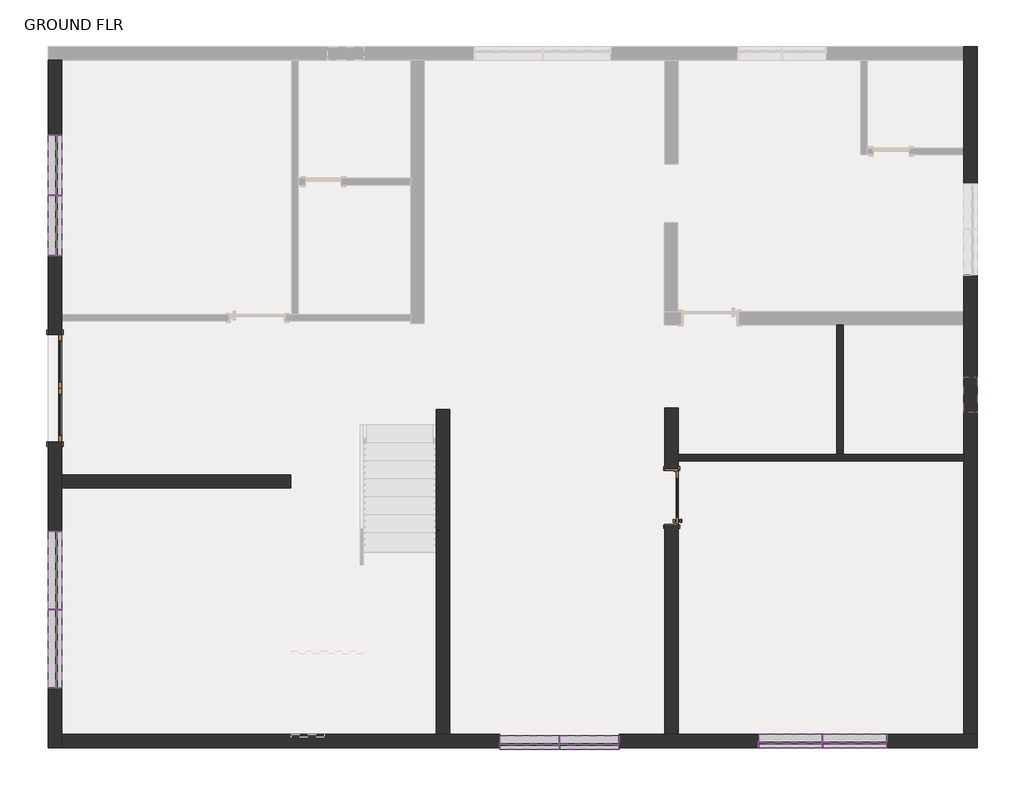
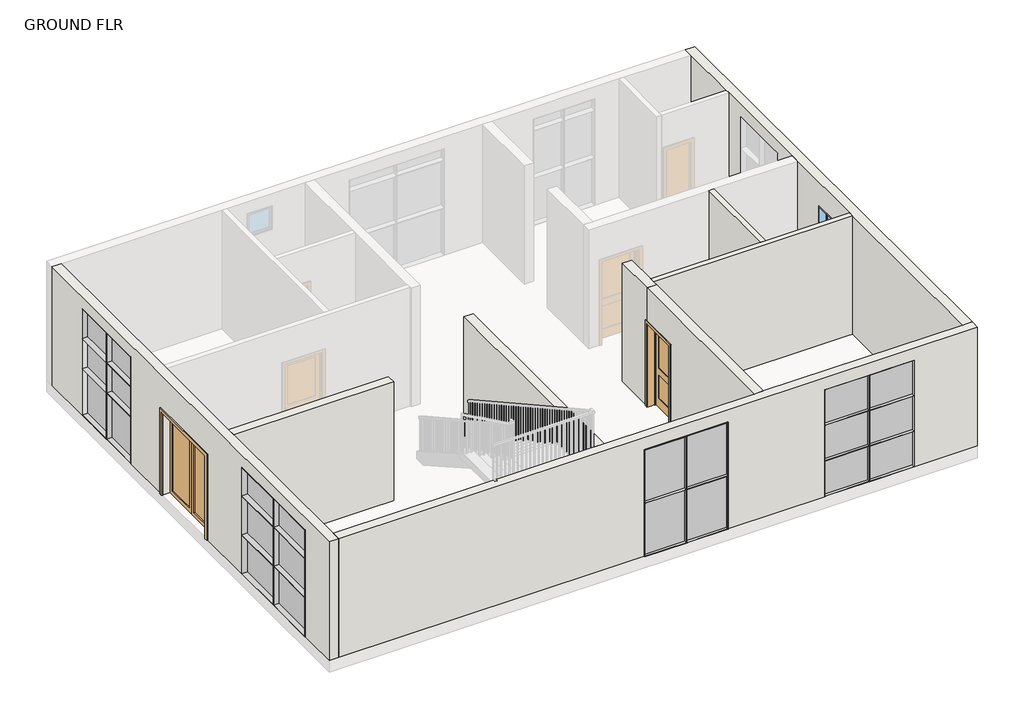
# One storey, part 1 of 3: 61 members, 22 plates, 9 walls, 2 doors, 1 window.
"""IFC4 building model written with IfcOpenShell, lengths in millimetres."""

from ifc_helpers import new_model, si_unit, frame, origin, place, context, project, spatial, polyline, outline, extrude, faceted_brep, transform, mapped, element, save
from components import door_5cbd26dd, door_interior_single_2_panel_wood_5dd36918, member_897fe9bb, member_9b8c6d2b, member_2938acba, member_330b65be, member_3bd50dc0, member_3448d7e6, member_1c5a217c, member_cd12fca0, member_0b5c0894, member_065c0f10, member_eaa18777, member_15c0e2f7, member_46601aaa, member_1d4720dc, member_9e0b9b87, member_6fc4240e, member_2d61f393, member_06a73730, member_9004b0e6, member_781c77f6, system_panel_glazed_9c96ef9a, system_panel_glazed_c3157265, system_panel_glazed_1bc24549, system_panel_glazed_9cc9ac89, system_panel_glazed_cb69acbc, system_panel_glazed_51d5fa28, system_panel_glazed_d128e385, system_panel_glazed_c2edcddf, system_panel_glazed_7a42c5f5, window_80340324

model = new_model("IFC4")

# Units and contexts
model_context = context("Model", 3, world=origin())
ifc_project = project(units=[si_unit("LENGTHUNIT", "METRE", prefix="MILLI")], contexts=[model_context])

# Site, building, storey
site = spatial("IfcSite", under=ifc_project)
building = spatial("IfcBuilding", under=site)
storey = spatial("IfcBuildingStorey", under=building, Name="GROUND FLR", Elevation=304.8)

# Doors
placement = place(None, origin())
door_shape = door_5cbd26dd(model_context)
element("IfcDoor", 1, ObjectType="Door-Double-Glass : 72\" x 84\"", at=placement, inside=storey, context=model_context, shape_type="MappedRepresentation", body=[
    mapped(door_shape, transform((-10241.447001, -123.3828332, 304.8), x_axis=(0.0, -1.0, 0.0), y_axis=(1.0, 0.0, 0.0), z_axis=(0.0, 0.0, 1.0))),
])
door_interior_single_2_panel_wood_shape = door_interior_single_2_panel_wood_5dd36918(model_context)
element("IfcDoor", 2, ObjectType="Door-Interior-Single-2_Panel-Wood", at=placement, inside=storey, context=model_context, shape_type="MappedRepresentation", body=[
    mapped(door_interior_single_2_panel_wood_shape, transform((226.2108119, -1978.5424275, 304.8), x_axis=(0.0, 1.0, 0.0), y_axis=(-1.0, 0.0, 0.0), z_axis=(0.0, 0.0, 1.0))),
])

# Members
member_shape = member_897fe9bb(model_context)
element("IfcMember", 3, ObjectType="Rectangular Mullion : 2.5\" x 5\" rectangular", at=placement, inside=storey, context=model_context, shape_type="MappedRepresentation", body=[
    mapped(member_shape, transform((-10239.065751, 3150.98206, 304.8), x_axis=(0.0, -1.0, 0.0), y_axis=(-1.0, 0.0, 0.0), z_axis=(0.0, 0.0, -1.0))),
])
member_2_shape = member_9b8c6d2b(model_context)
element("IfcMember", 4, ObjectType="Rectangular Mullion : 2.5\" x 5\" rectangular", at=placement, inside=storey, context=model_context, shape_type="MappedRepresentation", body=[
    mapped(member_2_shape, transform((-10239.065751, 2122.28206, 304.8), x_axis=(0.0, -1.0, 0.0), y_axis=(-1.0, 0.0, 0.0), z_axis=(0.0, 0.0, -1.0))),
])
member_3_shape = member_2938acba(model_context)
element("IfcMember", 5, ObjectType="Rectangular Mullion : 2.5\" x 5\" rectangular", at=placement, inside=storey, context=model_context, shape_type="MappedRepresentation", body=[
    mapped(member_3_shape, transform((-10239.065751, 3150.98206, 1498.6), x_axis=(0.0, -1.0, 0.0), y_axis=(-1.0, 0.0, 0.0), z_axis=(0.0, 0.0, -1.0))),
])
element("IfcMember", 6, ObjectType="Rectangular Mullion : 2.5\" x 5\" rectangular", at=placement, inside=storey, context=model_context, shape_type="MappedRepresentation", body=[
    mapped(member_3_shape, transform((-10239.065751, 3150.98206, 2273.3), x_axis=(0.0, -1.0, 0.0), y_axis=(-1.0, 0.0, 0.0), z_axis=(0.0, 0.0, -1.0))),
])
member_4_shape = member_330b65be(model_context)
element("IfcMember", 7, ObjectType="Rectangular Mullion : 2.5\" x 5\" rectangular", at=placement, inside=storey, context=model_context, shape_type="MappedRepresentation", body=[
    mapped(member_4_shape, transform((-10239.065751, 4179.68206, 3048.0), x_axis=(0.0, 1.0, 0.0), y_axis=(-1.0, 0.0, 0.0), z_axis=(0.0, 0.0, 1.0))),
])
element("IfcMember", 8, ObjectType="Rectangular Mullion : 2.5\" x 5\" rectangular", at=placement, inside=storey, context=model_context, shape_type="MappedRepresentation", body=[
    mapped(member_4_shape, transform((-10239.065751, 2122.28206, 1498.6), x_axis=(0.0, -1.0, 0.0), y_axis=(-1.0, 0.0, 0.0), z_axis=(0.0, 0.0, -1.0))),
])
element("IfcMember", 9, ObjectType="Rectangular Mullion : 2.5\" x 5\" rectangular", at=placement, inside=storey, context=model_context, shape_type="MappedRepresentation", body=[
    mapped(member_4_shape, transform((-10239.065751, 2122.28206, 2273.3), x_axis=(0.0, -1.0, 0.0), y_axis=(-1.0, 0.0, 0.0), z_axis=(0.0, 0.0, -1.0))),
])
member_5_shape = member_3bd50dc0(model_context)
element("IfcMember", 10, ObjectType="Rectangular Mullion : 2.5\" x 5\" rectangular", at=placement, inside=storey, context=model_context, shape_type="MappedRepresentation", body=[
    mapped(member_5_shape, transform((-10239.065751, -3879.168209, 2311.4), x_axis=(0.0, -1.0, 0.0), y_axis=(-1.0, 0.0, 0.0), z_axis=(0.0, 0.0, -1.0))),
])
member_6_shape = member_3448d7e6(model_context)
element("IfcMember", 11, ObjectType="Rectangular Mullion : 2.5\" x 5\" rectangular", at=placement, inside=storey, context=model_context, shape_type="MappedRepresentation", body=[
    mapped(member_6_shape, transform((-10239.065751, -2545.668209, 3048.0), x_axis=(0.0, 1.0, 0.0), y_axis=(-1.0, 0.0, 0.0), z_axis=(0.0, 0.0, 1.0))),
])
element("IfcMember", 12, ObjectType="Rectangular Mullion : 2.5\" x 5\" rectangular", at=placement, inside=storey, context=model_context, shape_type="MappedRepresentation", body=[
    mapped(member_6_shape, transform((-10239.065751, -5212.668209, 2311.4), x_axis=(0.0, -1.0, 0.0), y_axis=(-1.0, 0.0, 0.0), z_axis=(0.0, 0.0, -1.0))),
])
member_7_shape = member_1c5a217c(model_context)
element("IfcMember", 13, ObjectType="Rectangular Mullion : 2.5\" x 5\" rectangular", at=placement, inside=storey, context=model_context, shape_type="MappedRepresentation", body=[
    mapped(member_7_shape, transform((-10239.065751, -3879.168209, 304.8), x_axis=(0.0, -1.0, 0.0), y_axis=(-1.0, 0.0, 0.0), z_axis=(0.0, 0.0, -1.0))),
])
element("IfcMember", 14, ObjectType="Rectangular Mullion : 2.5\" x 5\" rectangular", at=placement, inside=storey, context=model_context, shape_type="MappedRepresentation", body=[
    mapped(member_7_shape, transform((-10239.065751, -3879.168209, 1308.1), x_axis=(0.0, -1.0, 0.0), y_axis=(-1.0, 0.0, 0.0), z_axis=(0.0, 0.0, -1.0))),
])
member_8_shape = member_cd12fca0(model_context)
element("IfcMember", 15, ObjectType="Rectangular Mullion : 2.5\" x 5\" rectangular", at=placement, inside=storey, context=model_context, shape_type="MappedRepresentation", body=[
    mapped(member_8_shape, transform((-10239.065751, -5212.668209, 304.8), x_axis=(0.0, -1.0, 0.0), y_axis=(-1.0, 0.0, 0.0), z_axis=(0.0, 0.0, -1.0))),
])
element("IfcMember", 16, ObjectType="Rectangular Mullion : 2.5\" x 5\" rectangular", at=placement, inside=storey, context=model_context, shape_type="MappedRepresentation", body=[
    mapped(member_8_shape, transform((-10239.065751, -2545.668209, 2311.4), x_axis=(0.0, 1.0, 0.0), y_axis=(-1.0, 0.0, 0.0), z_axis=(0.0, 0.0, 1.0))),
])
element("IfcMember", 17, ObjectType="Rectangular Mullion : 2.5\" x 5\" rectangular", at=placement, inside=storey, context=model_context, shape_type="MappedRepresentation", body=[
    mapped(member_8_shape, transform((-10239.065751, -5212.668209, 1308.1), x_axis=(0.0, -1.0, 0.0), y_axis=(-1.0, 0.0, 0.0), z_axis=(0.0, 0.0, -1.0))),
])
element("IfcMember", 18, ObjectType="Rectangular Mullion : 2.5\" x 5\" rectangular", at=placement, inside=storey, context=model_context, shape_type="MappedRepresentation", body=[
    mapped(member_8_shape, transform((-10239.065751, -2545.668209, 1308.1), x_axis=(0.0, 1.0, 0.0), y_axis=(-1.0, 0.0, 0.0), z_axis=(0.0, 0.0, 1.0))),
])
member_9_shape = member_0b5c0894(model_context)
element("IfcMember", 19, ObjectType="Rectangular Mullion : 2.5\" x 5\" rectangular", at=placement, inside=storey, context=model_context, shape_type="MappedRepresentation", body=[
    mapped(member_9_shape, transform((2781.5067356, -6110.4053142, 2133.6), x_axis=(-1.0, 0.0, 0.0), y_axis=(0.0, 1.0, 0.0), z_axis=(0.0, 0.0, -1.0))),
])
member_10_shape = member_065c0f10(model_context)
element("IfcMember", 20, ObjectType="Rectangular Mullion : 2.5\" x 5\" rectangular", at=placement, inside=storey, context=model_context, shape_type="MappedRepresentation", body=[
    mapped(member_10_shape, transform((3873.7067356, -6110.4053142, 3048.0), x_axis=(1.0, 0.0, 0.0), y_axis=(0.0, 1.0, 0.0), z_axis=(0.0, 0.0, 1.0))),
])
element("IfcMember", 21, ObjectType="Rectangular Mullion : 2.5\" x 5\" rectangular", at=placement, inside=storey, context=model_context, shape_type="MappedRepresentation", body=[
    mapped(member_10_shape, transform((1689.3067356, -6110.4053142, 2133.6), x_axis=(-1.0, 0.0, 0.0), y_axis=(0.0, 1.0, 0.0), z_axis=(0.0, 0.0, -1.0))),
])
element("IfcMember", 22, ObjectType="Rectangular Mullion : 2.5\" x 5\" rectangular", at=placement, inside=storey, context=model_context, shape_type="MappedRepresentation", body=[
    mapped(member_9_shape, transform((2781.5067356, -6110.4053142, 304.8), x_axis=(-1.0, 0.0, 0.0), y_axis=(0.0, 1.0, 0.0), z_axis=(0.0, 0.0, -1.0))),
])
element("IfcMember", 23, ObjectType="Rectangular Mullion : 2.5\" x 5\" rectangular", at=placement, inside=storey, context=model_context, shape_type="MappedRepresentation", body=[
    mapped(member_9_shape, transform((2781.5067356, -6110.4053142, 1219.2), x_axis=(-1.0, 0.0, 0.0), y_axis=(0.0, 1.0, 0.0), z_axis=(0.0, 0.0, -1.0))),
])
element("IfcMember", 24, ObjectType="Rectangular Mullion : 2.5\" x 5\" rectangular", at=placement, inside=storey, context=model_context, shape_type="MappedRepresentation", body=[
    mapped(member_10_shape, transform((1689.3067356, -6110.4053142, 304.8), x_axis=(-1.0, 0.0, 0.0), y_axis=(0.0, 1.0, 0.0), z_axis=(0.0, 0.0, -1.0))),
])
element("IfcMember", 25, ObjectType="Rectangular Mullion : 2.5\" x 5\" rectangular", at=placement, inside=storey, context=model_context, shape_type="MappedRepresentation", body=[
    mapped(member_10_shape, transform((3873.7067356, -6110.4053142, 2133.6), x_axis=(1.0, 0.0, 0.0), y_axis=(0.0, 1.0, 0.0), z_axis=(0.0, 0.0, 1.0))),
])
element("IfcMember", 26, ObjectType="Rectangular Mullion : 2.5\" x 5\" rectangular", at=placement, inside=storey, context=model_context, shape_type="MappedRepresentation", body=[
    mapped(member_10_shape, transform((1689.3067356, -6110.4053142, 1219.2), x_axis=(-1.0, 0.0, 0.0), y_axis=(0.0, 1.0, 0.0), z_axis=(0.0, 0.0, -1.0))),
])
element("IfcMember", 27, ObjectType="Rectangular Mullion : 2.5\" x 5\" rectangular", at=placement, inside=storey, context=model_context, shape_type="MappedRepresentation", body=[
    mapped(member_10_shape, transform((3873.7067356, -6110.4053142, 1219.2), x_axis=(1.0, 0.0, 0.0), y_axis=(0.0, 1.0, 0.0), z_axis=(0.0, 0.0, 1.0))),
])
member_11_shape = member_eaa18777(model_context)
element("IfcMember", 28, ObjectType="Rectangular Mullion : 2.5\" x 5\" rectangular", at=placement, inside=storey, context=model_context, shape_type="MappedRepresentation", body=[
    mapped(member_11_shape, transform((-1680.5487435, -6133.1318323, 304.8), x_axis=(-1.0, 0.0, 0.0), y_axis=(0.0, 1.0, 0.0), z_axis=(0.0, 0.0, -1.0))),
])
element("IfcMember", 29, ObjectType="Rectangular Mullion : 2.5\" x 5\" rectangular", at=placement, inside=storey, context=model_context, shape_type="MappedRepresentation", body=[
    mapped(member_11_shape, transform((-1680.5487435, -6133.1318323, 1676.4), x_axis=(-1.0, 0.0, 0.0), y_axis=(0.0, 1.0, 0.0), z_axis=(0.0, 0.0, -1.0))),
])
member_12_shape = member_15c0e2f7(model_context)
element("IfcMember", 30, ObjectType="Rectangular Mullion : 2.5\" x 5\" rectangular", at=placement, inside=storey, context=model_context, shape_type="MappedRepresentation", body=[
    mapped(member_12_shape, transform((-2696.5487435, -6133.1318323, 304.8), x_axis=(-1.0, 0.0, 0.0), y_axis=(0.0, 1.0, 0.0), z_axis=(0.0, 0.0, -1.0))),
])
element("IfcMember", 31, ObjectType="Rectangular Mullion : 2.5\" x 5\" rectangular", at=placement, inside=storey, context=model_context, shape_type="MappedRepresentation", body=[
    mapped(member_12_shape, transform((-664.5487435, -6133.1318323, 3048.0), x_axis=(1.0, 0.0, 0.0), y_axis=(0.0, 1.0, 0.0), z_axis=(0.0, 0.0, 1.0))),
])
element("IfcMember", 32, ObjectType="Rectangular Mullion : 2.5\" x 5\" rectangular", at=placement, inside=storey, context=model_context, shape_type="MappedRepresentation", body=[
    mapped(member_12_shape, transform((-2696.5487435, -6133.1318323, 1676.4), x_axis=(-1.0, 0.0, 0.0), y_axis=(0.0, 1.0, 0.0), z_axis=(0.0, 0.0, -1.0))),
])
element("IfcMember", 33, ObjectType="Rectangular Mullion : 2.5\" x 5\" rectangular", at=placement, inside=storey, context=model_context, shape_type="MappedRepresentation", body=[
    mapped(member_12_shape, transform((-664.5487435, -6133.1318323, 1676.4), x_axis=(1.0, 0.0, 0.0), y_axis=(0.0, 1.0, 0.0), z_axis=(0.0, 0.0, 1.0))),
])
member_13_shape = member_46601aaa(model_context)
element("IfcMember", 34, ObjectType="Rectangular Mullion : 2.5\" x 5\" rectangular", at=placement, inside=storey, context=model_context, shape_type="MappedRepresentation", body=[
    mapped(member_13_shape, transform((-10239.065751, 2129.52106, 3048.0), x_axis=(0.0, 0.0, 1.0), y_axis=(-1.0, 0.0, 0.0), z_axis=(0.0, -1.0, 0.0))),
])
element("IfcMember", 35, ObjectType="Rectangular Mullion : 2.5\" x 5\" rectangular", at=placement, inside=storey, context=model_context, shape_type="MappedRepresentation", body=[
    mapped(member_13_shape, transform((-10239.065751, 3154.60156, 3048.0), x_axis=(0.0, 0.0, 1.0), y_axis=(-1.0, 0.0, 0.0), z_axis=(0.0, -1.0, 0.0))),
])
element("IfcMember", 36, ObjectType="Rectangular Mullion : 2.5\" x 5\" rectangular", at=placement, inside=storey, context=model_context, shape_type="MappedRepresentation", body=[
    mapped(member_13_shape, transform((-10239.065751, 4172.44306, 304.8), x_axis=(0.0, 0.0, -1.0), y_axis=(-1.0, 0.0, 0.0), z_axis=(0.0, 1.0, 0.0))),
])
element("IfcMember", 37, ObjectType="Rectangular Mullion : 2.5\" x 5\" rectangular", at=placement, inside=storey, context=model_context, shape_type="MappedRepresentation", body=[
    mapped(member_13_shape, transform((-10239.065751, 3147.36256, 304.8), x_axis=(0.0, 0.0, -1.0), y_axis=(-1.0, 0.0, 0.0), z_axis=(0.0, 1.0, 0.0))),
])
member_14_shape = member_1d4720dc(model_context)
element("IfcMember", 38, ObjectType="Rectangular Mullion : 2.5\" x 5\" rectangular", at=placement, inside=storey, context=model_context, shape_type="MappedRepresentation", body=[
    mapped(member_14_shape, transform((-10239.065751, 3154.60156, 1498.6), x_axis=(0.0, 0.0, 1.0), y_axis=(-1.0, 0.0, 0.0), z_axis=(0.0, -1.0, 0.0))),
])
element("IfcMember", 39, ObjectType="Rectangular Mullion : 2.5\" x 5\" rectangular", at=placement, inside=storey, context=model_context, shape_type="MappedRepresentation", body=[
    mapped(member_14_shape, transform((-10239.065751, 2129.52106, 1498.6), x_axis=(0.0, 0.0, 1.0), y_axis=(-1.0, 0.0, 0.0), z_axis=(0.0, -1.0, 0.0))),
])
element("IfcMember", 40, ObjectType="Rectangular Mullion : 2.5\" x 5\" rectangular", at=placement, inside=storey, context=model_context, shape_type="MappedRepresentation", body=[
    mapped(member_14_shape, transform((-10239.065751, 3154.60156, 2273.3), x_axis=(0.0, 0.0, 1.0), y_axis=(-1.0, 0.0, 0.0), z_axis=(0.0, -1.0, 0.0))),
])
element("IfcMember", 41, ObjectType="Rectangular Mullion : 2.5\" x 5\" rectangular", at=placement, inside=storey, context=model_context, shape_type="MappedRepresentation", body=[
    mapped(member_14_shape, transform((-10239.065751, 2129.52106, 2273.3), x_axis=(0.0, 0.0, 1.0), y_axis=(-1.0, 0.0, 0.0), z_axis=(0.0, -1.0, 0.0))),
])
member_15_shape = member_9e0b9b87(model_context)
element("IfcMember", 42, ObjectType="Rectangular Mullion : 2.5\" x 5\" rectangular", at=placement, inside=storey, context=model_context, shape_type="MappedRepresentation", body=[
    mapped(member_15_shape, transform((-10239.065751, -5205.429209, 3048.0), x_axis=(0.0, 0.0, 1.0), y_axis=(-1.0, 0.0, 0.0), z_axis=(0.0, -1.0, 0.0))),
])
element("IfcMember", 43, ObjectType="Rectangular Mullion : 2.5\" x 5\" rectangular", at=placement, inside=storey, context=model_context, shape_type="MappedRepresentation", body=[
    mapped(member_15_shape, transform((-10239.065751, -3875.548709, 3048.0), x_axis=(0.0, 0.0, 1.0), y_axis=(-1.0, 0.0, 0.0), z_axis=(0.0, -1.0, 0.0))),
])
element("IfcMember", 44, ObjectType="Rectangular Mullion : 2.5\" x 5\" rectangular", at=placement, inside=storey, context=model_context, shape_type="MappedRepresentation", body=[
    mapped(member_15_shape, transform((-10239.065751, -2552.907209, 304.8), x_axis=(0.0, 0.0, -1.0), y_axis=(-1.0, 0.0, 0.0), z_axis=(0.0, 1.0, 0.0))),
])
element("IfcMember", 45, ObjectType="Rectangular Mullion : 2.5\" x 5\" rectangular", at=placement, inside=storey, context=model_context, shape_type="MappedRepresentation", body=[
    mapped(member_15_shape, transform((-10239.065751, -3882.787709, 304.8), x_axis=(0.0, 0.0, -1.0), y_axis=(-1.0, 0.0, 0.0), z_axis=(0.0, 1.0, 0.0))),
])
member_16_shape = member_6fc4240e(model_context)
element("IfcMember", 46, ObjectType="Rectangular Mullion : 2.5\" x 5\" rectangular", at=placement, inside=storey, context=model_context, shape_type="MappedRepresentation", body=[
    mapped(member_16_shape, transform((-10239.065751, -3875.548709, 2311.4), x_axis=(0.0, 0.0, 1.0), y_axis=(-1.0, 0.0, 0.0), z_axis=(0.0, -1.0, 0.0))),
])
element("IfcMember", 47, ObjectType="Rectangular Mullion : 2.5\" x 5\" rectangular", at=placement, inside=storey, context=model_context, shape_type="MappedRepresentation", body=[
    mapped(member_16_shape, transform((-10239.065751, -5205.429209, 2311.4), x_axis=(0.0, 0.0, 1.0), y_axis=(-1.0, 0.0, 0.0), z_axis=(0.0, -1.0, 0.0))),
])
element("IfcMember", 48, ObjectType="Rectangular Mullion : 2.5\" x 5\" rectangular", at=placement, inside=storey, context=model_context, shape_type="MappedRepresentation", body=[
    mapped(member_16_shape, transform((-10239.065751, -3875.548709, 1308.1), x_axis=(0.0, 0.0, 1.0), y_axis=(-1.0, 0.0, 0.0), z_axis=(0.0, -1.0, 0.0))),
])
element("IfcMember", 49, ObjectType="Rectangular Mullion : 2.5\" x 5\" rectangular", at=placement, inside=storey, context=model_context, shape_type="MappedRepresentation", body=[
    mapped(member_16_shape, transform((-10239.065751, -5205.429209, 1308.1), x_axis=(0.0, 0.0, 1.0), y_axis=(-1.0, 0.0, 0.0), z_axis=(0.0, -1.0, 0.0))),
])
member_17_shape = member_2d61f393(model_context)
element("IfcMember", 50, ObjectType="Rectangular Mullion : 2.5\" x 5\" rectangular", at=placement, inside=storey, context=model_context, shape_type="MappedRepresentation", body=[
    mapped(member_17_shape, transform((1696.5457356, -6110.4053142, 3048.0), x_axis=(0.0, 0.0, 1.0), y_axis=(0.0, 1.0, 0.0), z_axis=(-1.0, 0.0, 0.0))),
])
element("IfcMember", 51, ObjectType="Rectangular Mullion : 2.5\" x 5\" rectangular", at=placement, inside=storey, context=model_context, shape_type="MappedRepresentation", body=[
    mapped(member_17_shape, transform((2785.1262356, -6110.4053142, 3048.0), x_axis=(0.0, 0.0, 1.0), y_axis=(0.0, 1.0, 0.0), z_axis=(-1.0, 0.0, 0.0))),
])
element("IfcMember", 52, ObjectType="Rectangular Mullion : 2.5\" x 5\" rectangular", at=placement, inside=storey, context=model_context, shape_type="MappedRepresentation", body=[
    mapped(member_17_shape, transform((3866.4677356, -6110.4053142, 304.8), x_axis=(0.0, 0.0, -1.0), y_axis=(0.0, 1.0, 0.0), z_axis=(1.0, 0.0, 0.0))),
])
element("IfcMember", 53, ObjectType="Rectangular Mullion : 2.5\" x 5\" rectangular", at=placement, inside=storey, context=model_context, shape_type="MappedRepresentation", body=[
    mapped(member_17_shape, transform((2777.8872356, -6110.4053142, 304.8), x_axis=(0.0, 0.0, -1.0), y_axis=(0.0, 1.0, 0.0), z_axis=(1.0, 0.0, 0.0))),
])
member_18_shape = member_06a73730(model_context)
element("IfcMember", 54, ObjectType="Rectangular Mullion : 2.5\" x 5\" rectangular", at=placement, inside=storey, context=model_context, shape_type="MappedRepresentation", body=[
    mapped(member_18_shape, transform((2785.1262356, -6110.4053142, 2133.6), x_axis=(0.0, 0.0, 1.0), y_axis=(0.0, 1.0, 0.0), z_axis=(-1.0, 0.0, 0.0))),
])
element("IfcMember", 55, ObjectType="Rectangular Mullion : 2.5\" x 5\" rectangular", at=placement, inside=storey, context=model_context, shape_type="MappedRepresentation", body=[
    mapped(member_18_shape, transform((1696.5457356, -6110.4053142, 2133.6), x_axis=(0.0, 0.0, 1.0), y_axis=(0.0, 1.0, 0.0), z_axis=(-1.0, 0.0, 0.0))),
])
element("IfcMember", 56, ObjectType="Rectangular Mullion : 2.5\" x 5\" rectangular", at=placement, inside=storey, context=model_context, shape_type="MappedRepresentation", body=[
    mapped(member_18_shape, transform((2785.1262356, -6110.4053142, 1219.2), x_axis=(0.0, 0.0, 1.0), y_axis=(0.0, 1.0, 0.0), z_axis=(-1.0, 0.0, 0.0))),
])
element("IfcMember", 57, ObjectType="Rectangular Mullion : 2.5\" x 5\" rectangular", at=placement, inside=storey, context=model_context, shape_type="MappedRepresentation", body=[
    mapped(member_18_shape, transform((1696.5457356, -6110.4053142, 1219.2), x_axis=(0.0, 0.0, 1.0), y_axis=(0.0, 1.0, 0.0), z_axis=(-1.0, 0.0, 0.0))),
])
member_19_shape = member_9004b0e6(model_context)
element("IfcMember", 58, ObjectType="Rectangular Mullion : 2.5\" x 5\" rectangular", at=placement, inside=storey, context=model_context, shape_type="MappedRepresentation", body=[
    mapped(member_19_shape, transform((-2689.3097435, -6133.1318323, 3048.0), x_axis=(0.0, 0.0, 1.0), y_axis=(0.0, 1.0, 0.0), z_axis=(-1.0, 0.0, 0.0))),
])
element("IfcMember", 59, ObjectType="Rectangular Mullion : 2.5\" x 5\" rectangular", at=placement, inside=storey, context=model_context, shape_type="MappedRepresentation", body=[
    mapped(member_19_shape, transform((-1676.9292435, -6133.1318323, 3048.0), x_axis=(0.0, 0.0, 1.0), y_axis=(0.0, 1.0, 0.0), z_axis=(-1.0, 0.0, 0.0))),
])
element("IfcMember", 60, ObjectType="Rectangular Mullion : 2.5\" x 5\" rectangular", at=placement, inside=storey, context=model_context, shape_type="MappedRepresentation", body=[
    mapped(member_19_shape, transform((-671.7877435, -6133.1318323, 304.8), x_axis=(0.0, 0.0, -1.0), y_axis=(0.0, 1.0, 0.0), z_axis=(1.0, 0.0, 0.0))),
])
element("IfcMember", 61, ObjectType="Rectangular Mullion : 2.5\" x 5\" rectangular", at=placement, inside=storey, context=model_context, shape_type="MappedRepresentation", body=[
    mapped(member_19_shape, transform((-1684.1682435, -6133.1318323, 304.8), x_axis=(0.0, 0.0, -1.0), y_axis=(0.0, 1.0, 0.0), z_axis=(1.0, 0.0, 0.0))),
])
member_20_shape = member_781c77f6(model_context)
element("IfcMember", 62, ObjectType="Rectangular Mullion : 2.5\" x 5\" rectangular", at=placement, inside=storey, context=model_context, shape_type="MappedRepresentation", body=[
    mapped(member_20_shape, transform((-1676.9292435, -6133.1318323, 1676.4), x_axis=(0.0, 0.0, 1.0), y_axis=(0.0, 1.0, 0.0), z_axis=(-1.0, 0.0, 0.0))),
])
element("IfcMember", 63, ObjectType="Rectangular Mullion : 2.5\" x 5\" rectangular", at=placement, inside=storey, context=model_context, shape_type="MappedRepresentation", body=[
    mapped(member_20_shape, transform((-2689.3097435, -6133.1318323, 1676.4), x_axis=(0.0, 0.0, 1.0), y_axis=(0.0, 1.0, 0.0), z_axis=(-1.0, 0.0, 0.0))),
])

# Plates
system_panel_glazed_shape = system_panel_glazed_9c96ef9a(model_context)
element("IfcPlate", 64, ObjectType="System Panel : Glazed", at=placement, inside=storey, context=model_context, shape_type="MappedRepresentation", body=[
    mapped(system_panel_glazed_shape, transform((-10239.065751, 3663.52231, 312.039), x_axis=(0.0, -1.0, 0.0), y_axis=(1.0, 0.0, 0.0), z_axis=(0.0, 0.0, 1.0))),
])
element("IfcPlate", 65, ObjectType="System Panel : Glazed", at=placement, inside=storey, context=model_context, shape_type="MappedRepresentation", body=[
    mapped(system_panel_glazed_shape, transform((-10239.065751, 2638.44181, 312.039), x_axis=(0.0, -1.0, 0.0), y_axis=(1.0, 0.0, 0.0), z_axis=(0.0, 0.0, 1.0))),
])
system_panel_glazed_2_shape = system_panel_glazed_c3157265(model_context)
element("IfcPlate", 66, ObjectType="System Panel : Glazed", at=placement, inside=storey, context=model_context, shape_type="MappedRepresentation", body=[
    mapped(system_panel_glazed_2_shape, transform((-10239.065751, -3214.227959, 312.039), x_axis=(0.0, -1.0, 0.0), y_axis=(1.0, 0.0, 0.0), z_axis=(0.0, 0.0, 1.0))),
])
element("IfcPlate", 67, ObjectType="System Panel : Glazed", at=placement, inside=storey, context=model_context, shape_type="MappedRepresentation", body=[
    mapped(system_panel_glazed_2_shape, transform((-10239.065751, -4544.108459, 312.039), x_axis=(0.0, -1.0, 0.0), y_axis=(1.0, 0.0, 0.0), z_axis=(0.0, 0.0, 1.0))),
])
system_panel_glazed_3_shape = system_panel_glazed_1bc24549(model_context)
element("IfcPlate", 68, ObjectType="System Panel : Glazed", at=placement, inside=storey, context=model_context, shape_type="MappedRepresentation", body=[
    mapped(system_panel_glazed_3_shape, transform((3325.7969856, -6110.4053142, 312.039), x_axis=(-1.0, 0.0, 0.0), y_axis=(0.0, -1.0, 0.0), z_axis=(0.0, 0.0, 1.0))),
])
element("IfcPlate", 69, ObjectType="System Panel : Glazed", at=placement, inside=storey, context=model_context, shape_type="MappedRepresentation", body=[
    mapped(system_panel_glazed_3_shape, transform((2237.2164856, -6110.4053142, 312.039), x_axis=(-1.0, 0.0, 0.0), y_axis=(0.0, -1.0, 0.0), z_axis=(0.0, 0.0, 1.0))),
])
element("IfcPlate", 70, ObjectType="System Panel : Glazed", at=placement, inside=storey, context=model_context, shape_type="MappedRepresentation", body=[
    mapped(system_panel_glazed_3_shape, transform((3325.7969856, -6110.4053142, 2137.2195), x_axis=(-1.0, 0.0, 0.0), y_axis=(0.0, -1.0, 0.0), z_axis=(0.0, 0.0, 1.0))),
])
element("IfcPlate", 71, ObjectType="System Panel : Glazed", at=placement, inside=storey, context=model_context, shape_type="MappedRepresentation", body=[
    mapped(system_panel_glazed_3_shape, transform((2237.2164856, -6110.4053142, 2137.2195), x_axis=(-1.0, 0.0, 0.0), y_axis=(0.0, -1.0, 0.0), z_axis=(0.0, 0.0, 1.0))),
])
system_panel_glazed_4_shape = system_panel_glazed_9cc9ac89(model_context)
element("IfcPlate", 72, ObjectType="System Panel : Glazed", at=placement, inside=storey, context=model_context, shape_type="MappedRepresentation", body=[
    mapped(system_panel_glazed_4_shape, transform((-1174.3584935, -6133.1318323, 312.039), x_axis=(-1.0, 0.0, 0.0), y_axis=(0.0, -1.0, 0.0), z_axis=(0.0, 0.0, 1.0))),
])
element("IfcPlate", 73, ObjectType="System Panel : Glazed", at=placement, inside=storey, context=model_context, shape_type="MappedRepresentation", body=[
    mapped(system_panel_glazed_4_shape, transform((-2186.7389935, -6133.1318323, 312.039), x_axis=(-1.0, 0.0, 0.0), y_axis=(0.0, -1.0, 0.0), z_axis=(0.0, 0.0, 1.0))),
])
element("IfcPlate", 74, ObjectType="System Panel : Glazed", at=placement, inside=storey, context=model_context, shape_type="MappedRepresentation", body=[
    mapped(system_panel_glazed_4_shape, transform((-1174.3584935, -6133.1318323, 1680.0195), x_axis=(-1.0, 0.0, 0.0), y_axis=(0.0, -1.0, 0.0), z_axis=(0.0, 0.0, 1.0))),
])
element("IfcPlate", 75, ObjectType="System Panel : Glazed", at=placement, inside=storey, context=model_context, shape_type="MappedRepresentation", body=[
    mapped(system_panel_glazed_4_shape, transform((-2186.7389935, -6133.1318323, 1680.0195), x_axis=(-1.0, 0.0, 0.0), y_axis=(0.0, -1.0, 0.0), z_axis=(0.0, 0.0, 1.0))),
])
system_panel_glazed_5_shape = system_panel_glazed_cb69acbc(model_context)
element("IfcPlate", 76, ObjectType="System Panel : Glazed", at=placement, inside=storey, context=model_context, shape_type="MappedRepresentation", body=[
    mapped(system_panel_glazed_5_shape, transform((-10239.065751, 3663.52231, 1502.2195), x_axis=(0.0, -1.0, 0.0), y_axis=(1.0, 0.0, 0.0), z_axis=(0.0, 0.0, 1.0))),
])
element("IfcPlate", 77, ObjectType="System Panel : Glazed", at=placement, inside=storey, context=model_context, shape_type="MappedRepresentation", body=[
    mapped(system_panel_glazed_5_shape, transform((-10239.065751, 2638.44181, 1502.2195), x_axis=(0.0, -1.0, 0.0), y_axis=(1.0, 0.0, 0.0), z_axis=(0.0, 0.0, 1.0))),
])
system_panel_glazed_6_shape = system_panel_glazed_51d5fa28(model_context)
element("IfcPlate", 78, ObjectType="System Panel : Glazed", at=placement, inside=storey, context=model_context, shape_type="MappedRepresentation", body=[
    mapped(system_panel_glazed_6_shape, transform((-10239.065751, 3663.52231, 2276.9195), x_axis=(0.0, -1.0, 0.0), y_axis=(1.0, 0.0, 0.0), z_axis=(0.0, 0.0, 1.0))),
])
element("IfcPlate", 79, ObjectType="System Panel : Glazed", at=placement, inside=storey, context=model_context, shape_type="MappedRepresentation", body=[
    mapped(system_panel_glazed_6_shape, transform((-10239.065751, 2638.44181, 2276.9195), x_axis=(0.0, -1.0, 0.0), y_axis=(1.0, 0.0, 0.0), z_axis=(0.0, 0.0, 1.0))),
])
system_panel_glazed_7_shape = system_panel_glazed_d128e385(model_context)
element("IfcPlate", 80, ObjectType="System Panel : Glazed", at=placement, inside=storey, context=model_context, shape_type="MappedRepresentation", body=[
    mapped(system_panel_glazed_7_shape, transform((-10239.065751, -3214.227959, 2315.0195), x_axis=(0.0, -1.0, 0.0), y_axis=(1.0, 0.0, 0.0), z_axis=(0.0, 0.0, 1.0))),
])
element("IfcPlate", 81, ObjectType="System Panel : Glazed", at=placement, inside=storey, context=model_context, shape_type="MappedRepresentation", body=[
    mapped(system_panel_glazed_7_shape, transform((-10239.065751, -4544.108459, 2315.0195), x_axis=(0.0, -1.0, 0.0), y_axis=(1.0, 0.0, 0.0), z_axis=(0.0, 0.0, 1.0))),
])
system_panel_glazed_8_shape = system_panel_glazed_c2edcddf(model_context)
element("IfcPlate", 82, ObjectType="System Panel : Glazed", at=placement, inside=storey, context=model_context, shape_type="MappedRepresentation", body=[
    mapped(system_panel_glazed_8_shape, transform((-10239.065751, -3214.227959, 1311.7195), x_axis=(0.0, -1.0, 0.0), y_axis=(1.0, 0.0, 0.0), z_axis=(0.0, 0.0, 1.0))),
])
element("IfcPlate", 83, ObjectType="System Panel : Glazed", at=placement, inside=storey, context=model_context, shape_type="MappedRepresentation", body=[
    mapped(system_panel_glazed_8_shape, transform((-10239.065751, -4544.108459, 1311.7195), x_axis=(0.0, -1.0, 0.0), y_axis=(1.0, 0.0, 0.0), z_axis=(0.0, 0.0, 1.0))),
])
system_panel_glazed_9_shape = system_panel_glazed_7a42c5f5(model_context)
element("IfcPlate", 84, ObjectType="System Panel : Glazed", at=placement, inside=storey, context=model_context, shape_type="MappedRepresentation", body=[
    mapped(system_panel_glazed_9_shape, transform((3325.7969856, -6110.4053142, 1222.8195), x_axis=(-1.0, 0.0, 0.0), y_axis=(0.0, -1.0, 0.0), z_axis=(0.0, 0.0, 1.0))),
])
element("IfcPlate", 85, ObjectType="System Panel : Glazed", at=placement, inside=storey, context=model_context, shape_type="MappedRepresentation", body=[
    mapped(system_panel_glazed_9_shape, transform((2237.2164856, -6110.4053142, 1222.8195), x_axis=(-1.0, 0.0, 0.0), y_axis=(0.0, -1.0, 0.0), z_axis=(0.0, 0.0, 1.0))),
])

# Walls
element("IfcWall", 86, at=placement, inside=storey, context=model_context, shape_type="Brep", body=[
    faceted_brep([(5407.334249, -6224.7053142, 3352.8), (-10124.765751, -6224.7053142, 3352.8), (-10124.765751, -6224.7053142, 304.8), (-2696.5487435, -6224.7053142, 304.8), (-2696.5487435, -6224.7053142, 3048.0), (-664.5487435, -6224.7053142, 3048.0), (-664.5487435, -6224.7053142, 304.8), (1689.3067356, -6224.7053142, 304.8), (1689.3067356, -6224.7053142, 3048.0), (3873.7067356, -6224.7053142, 3048.0), (3873.7067356, -6224.7053142, 304.8), (5407.334249, -6224.7053142, 304.8), (-10124.765751, -5996.1053142, 3352.8), (-3766.7446058, -5996.1053142, 3352.8), (-3538.1446058, -5996.1053142, 3352.8), (108.7358119, -5996.1053142, 3352.8), (337.3358119, -5996.1053142, 3352.8), (5178.734249, -5996.1053142, 3352.8), (5407.334249, -5996.1053142, 3352.8), (5407.334249, -5996.1053142, 304.8), (5178.734249, -5996.1053142, 304.8), (3873.7067356, -5996.1053142, 304.8), (3873.7067356, -5996.1053142, 3048.0), (1689.3067356, -5996.1053142, 3048.0), (1689.3067356, -5996.1053142, 304.8), (337.3358119, -5996.1053142, 304.8), (108.7358119, -5996.1053142, 304.8), (-664.5487435, -5996.1053142, 304.8), (-664.5487435, -5996.1053142, 3048.0), (-2696.5487435, -5996.1053142, 3048.0), (-2696.5487435, -5996.1053142, 304.8), (-3538.1446058, -5996.1053142, 304.8), (-3766.7446058, -5996.1053142, 304.8), (-10124.765751, -5996.1053142, 304.8)], [[[0, 1, 2, 3, 4, 5, 6, 7, 8, 9, 10, 11]], [[12, 13, 14, 15, 16, 17, 18, 19, 20, 21, 22, 23, 24, 25, 26, 27, 28, 29, 30, 31, 32, 33]], [[19, 11, 10, 21, 20]], [[2, 33, 32, 31, 30, 3]], [[24, 7, 6, 27, 26, 25]], [[1, 0, 18, 17, 16, 15, 14, 13, 12]], [[0, 11, 19, 18]], [[2, 1, 12, 33]], [[9, 22, 21, 10]], [[22, 9, 8, 23]], [[23, 8, 7, 24]], [[5, 28, 27, 6]], [[28, 5, 4, 29]], [[29, 4, 3, 30]]]),
])
element("IfcWall", 87, at=placement, inside=storey, context=model_context, shape_type="Brep", body=[
    faceted_brep([(5407.334249, 5675.1946858, 3352.8), (5407.334249, -5996.1053142, 3352.8), (5407.334249, -5996.1053142, 304.8), (5407.334249, 1793.1596634, 304.8), (5407.334249, 1793.1596634, 3048.0), (5407.334249, 3348.9096634, 3048.0), (5407.334249, 3348.9096634, 304.8), (5407.334249, 5675.1946858, 304.8), (5407.334249, -538.3216798, 2743.2), (5407.334249, 71.2783202, 2743.2), (5407.334249, 71.2783202, 2133.6), (5407.334249, -538.3216798, 2133.6), (5178.734249, -5996.1053142, 3352.8), (5178.734249, -1357.4716798, 3352.8), (5178.734249, -1243.1716798, 3352.8), (5178.734249, 952.1551442, 3352.8), (5178.734249, 1180.7551442, 3352.8), (5178.734249, 3840.0446858, 3352.8), (5178.734249, 3954.3446858, 3352.8), (5178.734249, 5446.5946858, 3352.8), (5178.734249, 5675.1946858, 3352.8), (5178.734249, 5675.1946858, 304.8), (5178.734249, 5446.5946858, 304.8), (5178.734249, 3954.3446858, 304.8), (5178.734249, 3840.0446858, 304.8), (5178.734249, 3348.9096634, 304.8), (5178.734249, 3348.9096634, 3048.0), (5178.734249, 1793.1596634, 3048.0), (5178.734249, 1793.1596634, 304.8), (5178.734249, 1180.7551442, 304.8), (5178.734249, 952.1551442, 304.8), (5178.734249, -1243.1716798, 304.8), (5178.734249, -1357.4716798, 304.8), (5178.734249, -5996.1053142, 304.8), (5178.734249, -538.3216798, 2743.2), (5178.734249, -538.3216798, 2133.6), (5178.734249, 71.2783202, 2133.6), (5178.734249, 71.2783202, 2743.2)], [[[0, 1, 2, 3, 4, 5, 6, 7], [8, 9, 10, 11]], [[12, 13, 14, 15, 16, 17, 18, 19, 20, 21, 22, 23, 24, 25, 26, 27, 28, 29, 30, 31, 32, 33], [34, 35, 36, 37]], [[2, 33, 32, 31, 30, 29, 28, 3]], [[21, 7, 6, 25, 24, 23, 22]], [[1, 0, 20, 19, 18, 17, 16, 15, 14, 13, 12]], [[2, 1, 12, 33]], [[0, 7, 21, 20]], [[5, 26, 25, 6]], [[26, 5, 4, 27]], [[27, 4, 3, 28]], [[35, 34, 8, 11]], [[36, 35, 11, 10]], [[37, 36, 10, 9]], [[34, 37, 9, 8]]]),
])
element("IfcWall", 88, at=placement, inside=storey, context=model_context, shape_type="Brep", body=[
    faceted_brep([(-10353.365751, -1037.7828332, 2438.4), (-10353.365751, -1037.7828332, 304.8), (-10353.365751, -2545.668209, 304.8), (-10353.365751, -2545.668209, 3048.0), (-10353.365751, -5212.668209, 3048.0), (-10353.365751, -5212.668209, 304.8), (-10353.365751, -6224.7053142, 304.8), (-10353.365751, -6224.7053142, 3352.8), (-10353.365751, 5446.5946858, 3352.8), (-10353.365751, 5446.5946858, 304.8), (-10353.365751, 4179.68206, 304.8), (-10353.365751, 4179.68206, 3048.0), (-10353.365751, 2122.28206, 3048.0), (-10353.365751, 2122.28206, 304.8), (-10353.365751, 791.0171668, 304.8), (-10353.365751, 791.0171668, 2438.4), (-10124.765751, -2545.668209, 304.8), (-10124.765751, -1818.9707851, 304.8), (-10124.765751, -1590.3707851, 304.8), (-10124.765751, -1037.7828332, 304.8), (-10124.765751, -1037.7828332, 2438.4), (-10124.765751, 791.0171668, 2438.4), (-10124.765751, 791.0171668, 304.8), (-10124.765751, 1013.2671668, 304.8), (-10124.765751, 1127.5671668, 304.8), (-10124.765751, 2122.28206, 304.8), (-10124.765751, 2122.28206, 3048.0), (-10124.765751, 4179.68206, 3048.0), (-10124.765751, 4179.68206, 304.8), (-10124.765751, 5446.5946858, 304.8), (-10124.765751, 5446.5946858, 3352.8), (-10124.765751, 1127.5671668, 3352.8), (-10124.765751, 1013.2671668, 3352.8), (-10124.765751, -1590.3707851, 3352.8), (-10124.765751, -1818.9707851, 3352.8), (-10124.765751, -5996.1053142, 3352.8), (-10124.765751, -6224.7053142, 3352.8), (-10124.765751, -6224.7053142, 304.8), (-10124.765751, -5996.1053142, 304.8), (-10124.765751, -5212.668209, 304.8), (-10124.765751, -5212.668209, 3048.0), (-10124.765751, -2545.668209, 3048.0)], [[[0, 1, 2, 3, 4, 5, 6, 7, 8, 9, 10, 11, 12, 13, 14, 15]], [[16, 17, 18, 19, 20, 21, 22, 23, 24, 25, 26, 27, 28, 29, 30, 31, 32, 33, 34, 35, 36, 37, 38, 39, 40, 41]], [[9, 29, 28, 10]], [[37, 6, 5, 39, 38]], [[14, 13, 25, 24, 23, 22]], [[2, 1, 19, 18, 17, 16]], [[8, 7, 36, 35, 34, 33, 32, 31, 30]], [[9, 8, 30, 29]], [[7, 6, 37, 36]], [[27, 11, 10, 28]], [[11, 27, 26, 12]], [[12, 26, 25, 13]], [[41, 3, 2, 16]], [[3, 41, 40, 4]], [[4, 40, 39, 5]], [[20, 19, 1, 0]], [[21, 20, 0, 15]], [[22, 21, 15, 14]]]),
])
element("IfcWall", 89, at=placement, inside=storey, context=model_context, shape_type="SweptSolid", body=[
    extrude(outline(polyline([(-6238.565751, -1818.9707851), (-10124.765751, -1818.9707851), (-10124.765751, -1590.3707851), (-6238.565751, -1590.3707851), (-6238.565751, -1818.9707851)])), frame((0.0, 0.0, 304.8), z_axis=(0.0, 0.0, 1.0), x_axis=(1.0, 0.0, 0.0)), (0.0, 0.0, 1.0), 3048.0),
])
element("IfcWall", 90, at=placement, inside=storey, context=model_context, shape_type="SweptSolid", body=[
    extrude(outline(polyline([(-3538.1446058, -484.3053142), (-3538.1446058, -5996.1053142), (-3766.7446058, -5996.1053142), (-3766.7446058, -484.3053142), (-3538.1446058, -484.3053142)])), frame((0.0, 0.0, 304.8), z_axis=(0.0, 0.0, 1.0), x_axis=(1.0, 0.0, 0.0)), (0.0, 0.0, 1.0), 3048.0),
])
element("IfcWall", 91, at=placement, inside=storey, context=model_context, shape_type="Brep", body=[
    faceted_brep([(108.7358119, -454.5424275, 304.8), (108.7358119, -1495.9424275, 304.8), (108.7358119, -1495.9424275, 2463.8), (108.7358119, -1495.9424275, 3352.8), (108.7358119, -454.5424275, 3352.8), (337.3358119, -454.5424275, 304.8), (337.3358119, -454.5424275, 3352.8), (337.3358119, -1243.1716798, 3352.8), (337.3358119, -1357.4716798, 3352.8), (337.3358119, -1495.9424275, 3352.8), (337.3358119, -1495.9424275, 2463.8), (337.3358119, -1495.9424275, 304.8), (337.3358119, -1357.4716798, 304.8), (337.3358119, -1243.1716798, 304.8)], [[[0, 1, 2, 3, 4]], [[5, 6, 7, 8, 9, 10, 11, 12, 13]], [[1, 0, 5, 13, 12, 11]], [[3, 2, 1, 11, 10, 9]], [[4, 3, 9, 8, 7, 6]], [[0, 4, 6, 5]]]),
])
element("IfcWall", 92, at=placement, inside=storey, context=model_context, shape_type="SweptSolid", body=[
    extrude(outline(polyline([(-5996.1053142, 3352.8), (-1495.9424275, 3352.8), (-1495.9424275, 2463.8), (-2461.1424275, 2463.8), (-2461.1424275, 304.8), (-5996.1053142, 304.8), (-5996.1053142, 3352.8)])), frame((108.7358119, 0.0, 0.0), z_axis=(1.0, 0.0, 0.0), x_axis=(0.0, 1.0, 0.0)), (0.0, 0.0, 1.0), 228.6),
])
element("IfcWall", 93, ObjectType="INTERIOR WALL THICKNESS 4.5\"", at=placement, inside=storey, context=model_context, shape_type="Brep", body=[
    faceted_brep([(5178.734249, -1243.1716798, 304.8), (3134.034249, -1243.1716798, 304.8), (3019.734249, -1243.1716798, 304.8), (337.3358119, -1243.1716798, 304.8), (337.3358119, -1243.1716798, 3352.8), (3019.734249, -1243.1716798, 3352.8), (3134.034249, -1243.1716798, 3352.8), (5178.734249, -1243.1716798, 3352.8), (5178.734249, -1357.4716798, 304.8), (5178.734249, -1357.4716798, 3352.8), (337.3358119, -1357.4716798, 3352.8), (337.3358119, -1357.4716798, 304.8)], [[[0, 1, 2, 3, 4, 5, 6, 7]], [[8, 9, 10, 11]], [[3, 2, 1, 0, 8, 11]], [[7, 6, 5, 4, 10, 9]], [[0, 7, 9, 8]], [[4, 3, 11, 10]]]),
])
element("IfcWall", 94, ObjectType="INTERIOR WALL THICKNESS 4.5\"", at=placement, inside=storey, context=model_context, shape_type="SweptSolid", body=[
    extrude(outline(polyline([(3019.734249, -1243.1716798), (3019.734249, 952.1551442), (3134.034249, 952.1551442), (3134.034249, -1243.1716798), (3019.734249, -1243.1716798)])), frame((0.0, 0.0, 304.8), z_axis=(0.0, 0.0, 1.0), x_axis=(1.0, 0.0, 0.0)), (0.0, 0.0, 1.0), 3048.0),
])

# Window
window_shape = window_80340324(model_context)
element("IfcWindow", 95, ObjectType="Fixed : 24\" x 24\"", at=placement, inside=storey, context=model_context, shape_type="MappedRepresentation", body=[
    mapped(window_shape, transform((5293.034249, -271.6216798, 1219.2), x_axis=(0.0, -1.0, 0.0), y_axis=(1.0, 0.0, 0.0), z_axis=(0.0, 0.0, 1.0))),
])

save(model, "model.ifc")

# Revit data of these elements
# Type "Door-Double-Glass : 72\" x 84\""
#   Type Mark = "13"
#   Construction Type Id = "opn-d45"
#   Assembly Code = "C1020"
#   Analytic Construction = "Wood frame, double glass door "
#   W = 3' - 0"
#   Thickness = 0' - 2"
#   Thermal Resistance (R) = 1.8150 (h·ft²·°F)/BTU
#   Swing Angle [instance default] = 90.00°
#   Heat Transfer Coefficient (U) = 0.5510 BTU/(h·ft²·°F)
#   Height = 7' - 0"
#   Bottom Rail = 0' - 4"
#   Top Rail = 0' - 4"
#   Stiles = 0' - 4"
#   Trim Projection = 0' - 1"
#   Trim Width = 0' - 3"
#   Width = 6' - 0"
#   Define Thermal Properties by = 1
#   Glazing = Glass
#   Panel Material = Wood - Birch - Solid Stained Light Low Gloss
#   Trim Material = Paint - Sienna
#   Visual Light Transmittance = 0
#   Solar Heat Gain Coefficient = 0
#   Function = (empty or 0)
#   Wall Closure = (empty or 0)
# Type "Door-Interior-Single-2_Panel-Wood"
#   Type Mark = "10"
#   Assembly Code = "C1020300"
#   Analytic Construction = "Wooden"
#   Top Rail = 0' - 4 11/16"
#   Thickness = 0' - 1 3/8"
#   Thermal Resistance (R) = 2.5876 (h·ft²·°F)/BTU
#   Swing Angle [instance default] = 90.00°
#   Stiles = 0' - 4 3/4"
#   Rough Width = 3' - 2"
#   Rough Height = 7' - 1"
#   Lock Rail = 0' - 7 1/2"
#   Height = 7' - 0"
#   Width = 3' - 0"
#   Heat Transfer Coefficient (U) = 0.3865 BTU/(h·ft²·°F)
#   Bottom Rail = 0' - 9 1/8"
#   Trim Material = Cherry
#   Panel Material = Cherry
#   Frame Material = Cherry
#   Door Handle Material = Aluminum
#   Visual Light Transmittance = 0
#   Solar Heat Gain Coefficient = 0
#   Wall Closure = (empty or 0)
#   Function = (empty or 0)
# Type "Rectangular Mullion : 2.5\" x 5\" rectangular"
#   built-in parameter 1007304 = 0.75 (stored number, unit not read)
#   built-in parameter 1007301 = 0.011875 (stored number, unit not read)
#   built-in parameter 1007300 = 0.011875 (stored number, unit not read)
# Type "System Panel : Glazed"
#   Construction Type Id = "GSP4R"
#   Analytic Construction = "1/8 in Pilkington single glazing"
#   Visual Light Transmittance = 0.9
#   Solar Heat Gain Coefficient = 0.86
#   Heat Transfer Coefficient (U) = 1.18115 BTU/(h·ft²·°F)
#   Define Thermal Properties by = 1
# Type
#   Assembly Code = "B2010"
#   Layers, outside or top first: 0' - 9" "BEIGE COLOUR" (function 1)
# Type "INTERIOR WALL THICKNESS 4.5\""
#   Assembly Code = "B2010"
#   Layers, outside or top first: 0' - 4 1/2" "BEIGE COLOUR" (function 1)
# Type "Fixed : 24\" x 24\""
#   Type Mark = "3"
#   Construction Type Id = "GSP4R"
#   Assembly Code = "B2020100"
#   Analytic Construction = "1/8 in Pilkington single glazing"
#   Visual Light Transmittance = 0.9
#   Solar Heat Gain Coefficient = 0.78
#   Heat Transfer Coefficient (U) = 0.6496 BTU/(h·ft²·°F)
#   Height = 2' - 0"
#   Default Sill Height = 3' - 0"
#   Width = 2' - 0"
#   Window Inset = 0' - 0 3/4"
#   Define Thermal Properties by = 1
#   Define Thermal Properties by = 1
#   Glass Pane Material = Glass
#   Sash Material = Sash
#   Wall Closure = (empty or 0)
# Element 1 (IfcDoor, "Door-Double-Glass : 72\" x 84\"")
#   Swing Angle = 90.00°
#   Phase Created = New Construction
#   Materials on its faces: "Wood - Birch - Solid Stained Light Low Gloss", "Paint - Sienna", "Glass"
# Element 2 (IfcDoor, "Door-Interior-Single-2_Panel-Wood")
#   Swing Angle = 90.00°
#   Phase Created = New Construction
#   Materials on its faces: "Cherry", "Aluminum"
# Elements 3, 4, 5, 6, 7, 8, 9, 10, 11, 12, 13, 14, 15, 16, 17, 18, 19, 20, 21, 22, 23, 24, 25, 26, 27, 28, 29, 30, 31, 32, 33, 34, 35, 36, 37, 38, 39, 40, 41, 42, 43, 44, 45, 46, 47, 48, 49, 50, 51, 52, 53, 54, 55, 56, 57, 58, 59, 60, 61, 62, 63 (IfcMember, "Rectangular Mullion : 2.5\" x 5\" rectangular")
#   Phase Created = New Construction
#   Materials on its faces: "WINDOW GLASS MATERIAL"
# Elements 64, 65, 66, 67, 68, 69, 70, 71, 72, 73, 74, 75, 76, 77, 78, 79, 80, 81, 82, 83, 84, 85 (IfcPlate, "System Panel : Glazed")
#   Phase Created = New Construction
#   Materials on its faces: "Glass"
# Elements 86, 87, 88, 89, 90, 91, 92 (IfcWall)
#   Top Offset = 0' - 0"
#   Base Offset = 0' - 0"
#   wall height = 10' - 0"
#   Phase Created = New Construction
#   Base Constraint = GROUND FLR
#   Top Constraint = FIRST FLR
#   Materials on its faces: "BEIGE COLOUR"
# Elements 93, 94 (IfcWall, "INTERIOR WALL THICKNESS 4.5\"")
#   Top Offset = 0' - 0"
#   Base Offset = 0' - 0"
#   wall height = 10' - 0"
#   Phase Created = New Construction
#   Base Constraint = GROUND FLR
#   Top Constraint = FIRST FLR
#   Materials on its faces: "BEIGE COLOUR"
# Element 95 (IfcWindow, "Fixed : 24\" x 24\"")
#   Mark = "2"
#   Phase Created = New Construction
#   Materials on its faces: "Sash", "Glass"
# Materials
#   "Glass": class "Glass", colour RGB 0 128 192, transparency 0.75, Description = "Soda Lime Glass", Cost = 0
#   "Wood - Birch - Solid Stained Light Low Gloss": class "Wood", colour RGB 210 159 95, transparency 0, Cost = 0
#   "Paint - Sienna": colour RGB 118 70 51, transparency 0, Cost = 0
#   "Cherry": class "Wood", colour RGB 226 177 128, transparency 0, Description = "Prunus Serotina", Cost = 0
#   "Aluminum": class "Metal", colour RGB 247 247 247, transparency 0, Description = "Aluminum 6061", Cost = 0
#   "BEIGE COLOUR": class "Generic", colour RGB 120 120 120, transparency 0, Cost = 0
#   "Sash": class "Wood", colour RGB 224 178 126, transparency 0, Cost = 0
#   "WINDOW GLASS MATERIAL": class "Generic", colour RGB 120 120 120, transparency 0, Cost = 0
